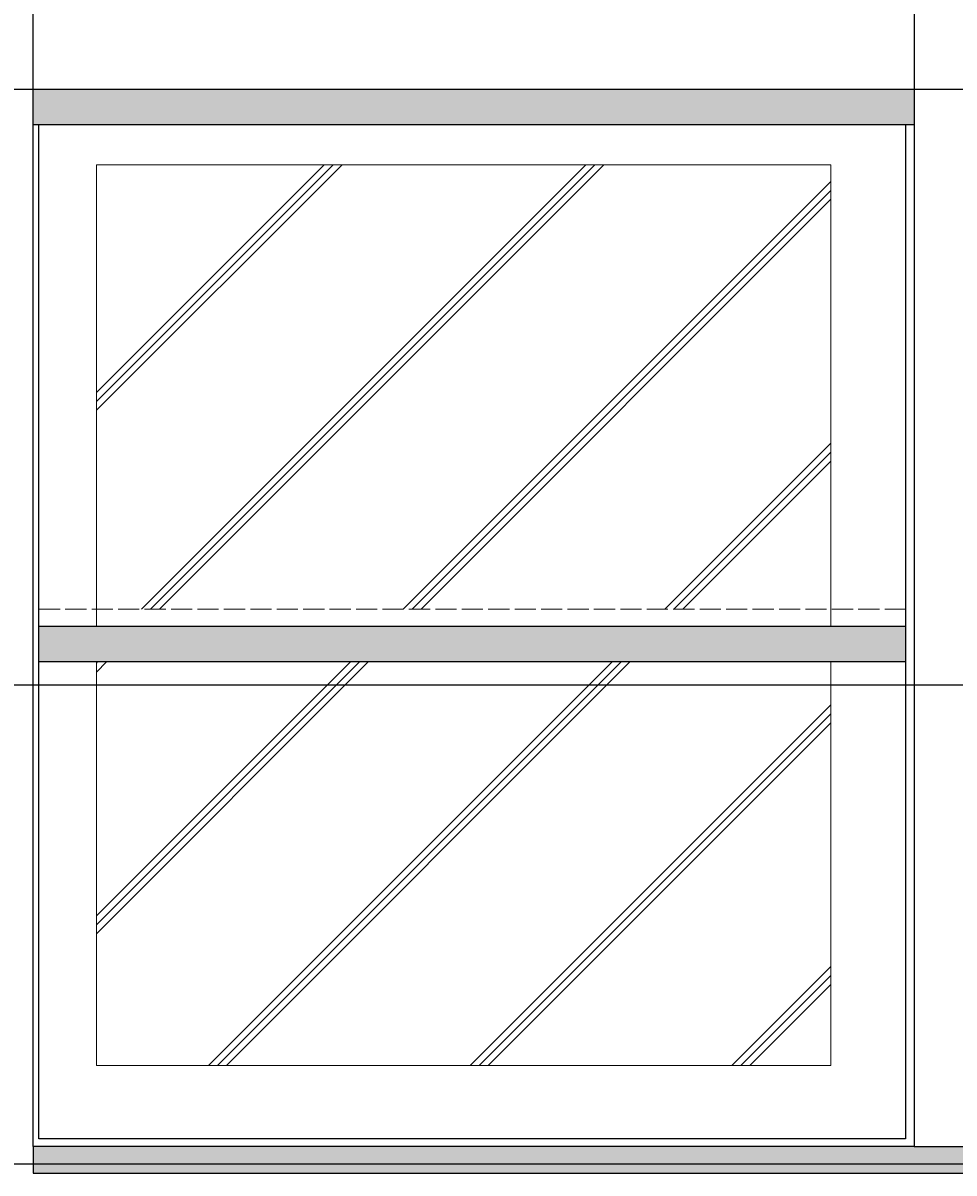
# Model space of a CAD drawing. Units: millimetres. Extents: x 2332 to 5836, y -853 to 2199.
# Tile 14 of 16: x 4779 to 5308, y 753 to 1405. Entities that reach past the tile are written whole.
import ezdxf

# ---------------------------------------------------------------- set-up
doc = ezdxf.new("R2010")
doc.units = ezdxf.units.MM
doc.linetypes.add('ACAD_ISO02W100', pattern=[15, 12, -3])
doc.layers.get('0').update_dxf_attribs({"color": 8})
for name, color, linetype, lineweight in [('A-ANNO-DIMS', 2, 'Continuous', 18), ('A-CSWK-GLAZ', 7, 'Continuous', 18), ('A-CSWK-HIDN', 8, 'ACAD_ISO02W100', 13), ('A-CSWK-PATT', 40, 'Continuous', 13), ('A-GLAZ-PATT', 4, 'Continuous', 13), ('SHELF', 40, 'Continuous', 25)]:
    doc.layers.add(name, color=color, linetype=linetype, lineweight=lineweight)
doc.styles.get("Standard").update_dxf_attribs({"font": 'arial.ttf'})
doc.dimstyles.new('ISO-25', dxfattribs={"dimtxt": 2.5, "dimasz": 2.5, "dimexe": 1.25, "dimexo": 0.625, "dimtad": 1, "dimtxsty": 'Standard', "dimcen": 2.5, "dimadec": 0, "dimazin": 0, "dimtfac": 1, "dimtmove": 0, "dimatfit": 3, "dimfxl": 1, "dimarcsym": 0})

# ---------------------------------------------------------------- blocks, each defined once
blk = doc.blocks.new('CAB-GLAZED-FACE-FRAME')
for p, q in [((500, 575.53), (0, 575.53)), ((5, 575.53), (5, 0)), ((496.71, 0), (496.71, 575.53)), ((5, 0), (496.71, 0))]:
    blk.add_line(p, q)
blk = doc.blocks.new('*D25')
at = {"layer": 'A-ANNO-DIMS', "color": 0, "lineweight": -2, "transparency": 16777216}
for p, q in [((4341.52, 1705.81), (5835.94, 1705.81)), ((5834.69, 1032.3), (5834.69, 1703.31)), ((4341.52, 1029.8), (5835.94, 1029.8))]:
    blk.add_line(p, q, dxfattribs=at)
at = {"layer": 'A-ANNO-DIMS', "color": 0, "transparency": 16777216}
for points in [[(5834.27, 1703.31), (5835.11, 1703.31), (5834.69, 1705.81)], [(5834.27, 1032.3), (5835.11, 1032.3), (5834.69, 1029.8)]]:
    blk.add_solid(points, dxfattribs=at)
at = {"layer": 'Defpoints', "color": 0, "transparency": 16777216}
for p in [(4340.89, 1705.81), (5834.69, 1705.81), (4340.89, 1029.8)]:
    blk.add_point(p, dxfattribs=at)
at = {"layer": 'A-ANNO-DIMS', "color": 0, "transparency": 16777216, "insert": (5832.79, 1367.8), "char_height": 2.5, "attachment_point": 5, "rotation": 90}
blk.add_mtext('676', dxfattribs=at)
blk = doc.blocks.new('*D26')
at = {"layer": 'A-ANNO-DIMS', "color": 0, "lineweight": -2, "transparency": 16777216}
for p, q in [((4774.24, 1029.8), (5835.94, 1029.8)), ((5834.69, 760.56), (5834.69, 1027.3)), ((4741.16, 758.06), (5835.94, 758.06))]:
    blk.add_line(p, q, dxfattribs=at)
at = {"layer": 'A-ANNO-DIMS', "color": 0, "transparency": 16777216}
for points in [[(5834.27, 1027.3), (5835.11, 1027.3), (5834.69, 1029.8)], [(5834.27, 760.56), (5835.11, 760.56), (5834.69, 758.06)]]:
    blk.add_solid(points, dxfattribs=at)
at = {"layer": 'Defpoints', "color": 0, "transparency": 16777216}
for p in [(4773.61, 1029.8), (5834.69, 1029.8), (4740.54, 758.06)]:
    blk.add_point(p, dxfattribs=at)
at = {"layer": 'A-ANNO-DIMS', "color": 0, "transparency": 16777216, "insert": (5832.81, 893.93), "char_height": 2.5, "attachment_point": 5, "rotation": 90}
blk.add_mtext('271.74', dxfattribs=at)

msp = doc.modelspace()

# ---------------------------------------------------------------- hatches: boundary and pattern name
at = {"layer": 'A-CSWK-PATT'}
h = msp.add_hatch(color=256, dxfattribs=at)
h.dxf.hatch_style = 1
h.paths.add_polyline_path([(4785.04, 1367.803), (5285.04, 1367.803), (5285.04, 1347.803), (4785.04, 1347.803)])
h.paths.add_polyline_path([(4821.011, 1062.803), (5237.731, 1062.803), (5237.731, 1042.803), (4821.011, 1042.803)])
h.paths.add_polyline_path([(5237.731, 1062.803), (5280.04, 1062.803), (5280.04, 1042.803), (5237.731, 1042.803)])
h.paths.add_polyline_path([(4788.33, 1062.803), (4821.011, 1062.803), (4821.011, 1042.803), (4788.33, 1042.803)])
h = msp.add_hatch(color=256, dxfattribs=at)
h.dxf.hatch_style = 1
h.paths.add_polyline_path([(4785.04, 767.803), (5285.04, 767.803), (5325.04, 767.803), (5621.17, 767.803), (5621.17, 752.803), (4785.04, 752.803)])
at = {"layer": 'A-GLAZ-PATT'}
h = msp.add_hatch(dxfattribs=at)
h.set_pattern_fill('JIS_RC_15', color=256, scale=7)
h.set_pattern_definition([(45, (210, 0), (-74.2462, 74.2462), []), (45, (215.07, 0), (-74.2462, 74.2462), []), (45, (220.15, 0), (-74.2462, 74.2462), [])])
h.paths.add_polyline_path([(4821.011, 1324.883), (4821.011, 1072.803), (5237.731, 1072.803), (5237.731, 1324.883)])
h.paths.add_polyline_path([(4821.011, 1042.803), (4821.011, 813.86), (5237.731, 813.86), (5237.731, 1042.803)])

# ---------------------------------------------------------------- linework, layer by layer
at = {"layer": 'A-CSWK-GLAZ'}
for points in [[(5237.731, 1062.803), (5237.731, 1324.883), (4821.011, 1324.883), (4821.011, 1062.803)], [(4821.011, 1042.803), (4821.011, 813.86), (5237.731, 813.86), (5237.731, 1042.803)]]:
    msp.add_lwpolyline(points, dxfattribs=at)
at = {"layer": 'A-CSWK-HIDN'}
msp.add_line((4788.33, 1072.803), (5280.04, 1072.803), dxfattribs=at)
at = {"layer": 'SHELF'}
for p, q in [((4785.04, 767.803), (4785.04, 1967.803)), ((5285.04, 1967.803), (5285.04, 767.803)), ((3635.04, 1367.803), (4785.04, 1367.803)), ((4785.04, 1367.803), (5675.04, 1367.803)), ((5280.04, 1062.803), (4788.33, 1062.803)), ((5280.04, 1042.803), (4788.33, 1042.803)), ((5285.04, 767.803), (4785.04, 767.803)), ((4785.04, 767.803), (4785.04, 752.803)), ((5285.04, 767.803), (5325.04, 767.803)), ((4785.04, 752.803), (5621.17, 752.803))]:
    msp.add_line(p, q, dxfattribs=at)

# ---------------------------------------------------------------- block references
at = {"layer": 'SHELF', "extrusion": (0, 0, -1), "zscale": -1}
msp.add_blockref('CAB-GLAZED-FACE-FRAME', (-5285.04, 772.269), dxfattribs=at)

# ---------------------------------------------------------------- dimensions: what is measured, and where the dimension line sits
at = {"layer": 'A-ANNO-DIMS'}
for base, p1, p2, override, picture, middle in [((5834.69, 1705.805), (4340.894, 1029.801), (4340.894, 1705.805), {"dimdec": 0, "dimlfac": 1, "dimrnd": 0, "dimzin": 0, "dimdsep": 46, "dimlunit": 2}, '*D25', (5832.788, 1367.803)), ((5834.69, 1029.801), (4740.539, 758.058), (4773.612, 1029.801), {"dimdec": 2, "dimlfac": 1, "dimrnd": 0, "dimzin": 0, "dimdsep": 46, "dimlunit": 2}, '*D26', (5832.81, 893.93))]:
    dim = msp.add_linear_dim(base=base, p1=p1, p2=p2, angle=90, dimstyle='ISO-25', override=override, dxfattribs=at)
    dim.commit()
    dim.dimension.update_dxf_attribs({"geometry": picture, "text_midpoint": middle})

doc.saveas('drawing.dxf')
